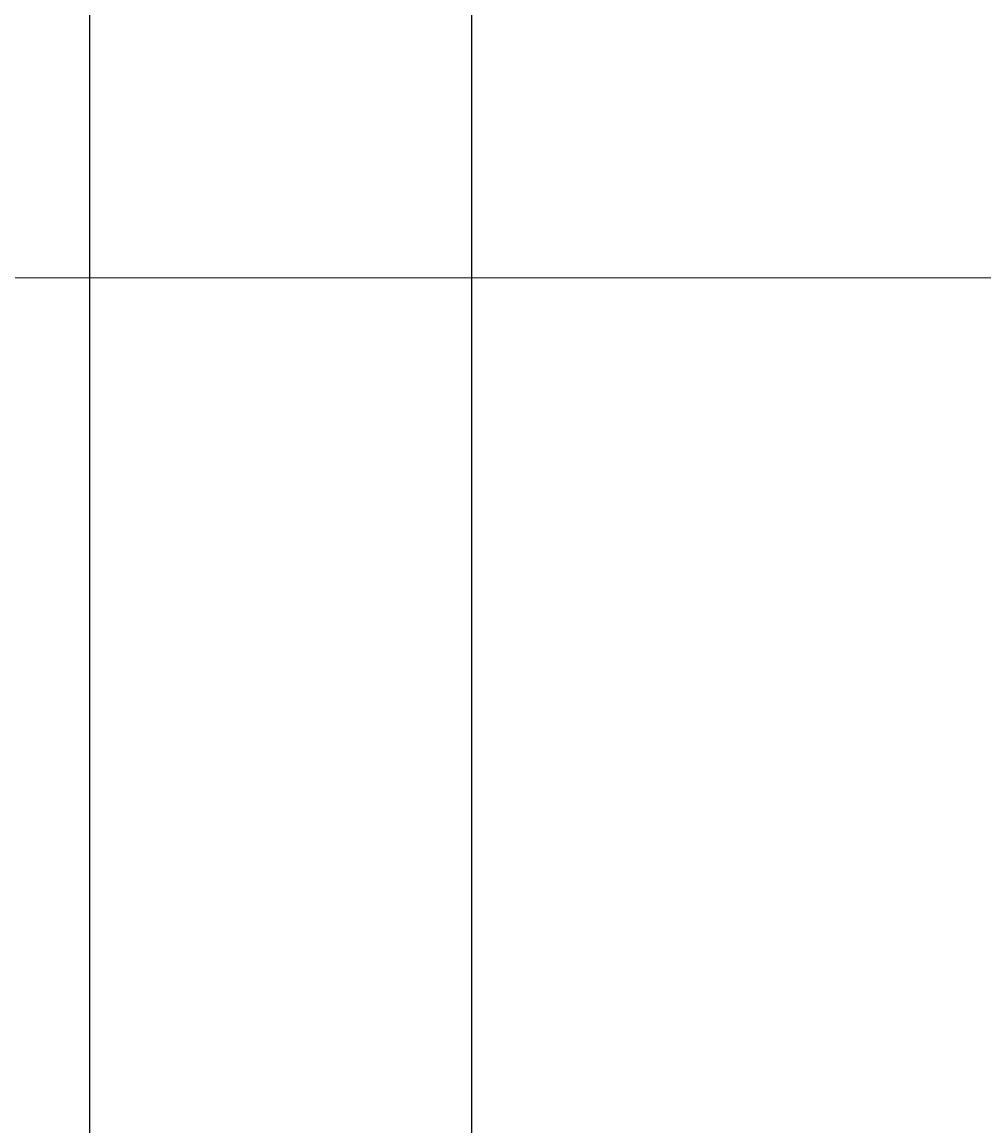
# Model space of a CAD drawing. Units: inches. Extents: x 738 to 1068, y 378 to 757.
# Tile 30 of 41: x 833 to 882, y 549 to 606. Entities that reach past the tile are written whole.
import ezdxf

# ---------------------------------------------------------------- set-up
doc = ezdxf.new("R2010")
doc.units = ezdxf.units.IN
doc.header["$MEASUREMENT"] = 0
doc.layers.add('A-ANNO-DIMS', color=2, linetype='Continuous', lineweight=18)
doc.layers.add('E-CTRL-WIRE', color=7, linetype='Continuous', lineweight=18)
doc.styles.get("Standard").update_dxf_attribs({"font": 'arial.ttf'})
doc.dimstyles.get("Standard").update_dxf_attribs({"dimtxt": 0.18, "dimasz": 0.18, "dimexe": 0.18, "dimexo": 0.0625, "dimgap": 0.09, "dimtad": 0, "dimtih": 1, "dimtoh": 1, "dimdec": 4, "dimzin": 0, "dimdsep": 46, "dimtxsty": 'Standard', "dimcen": 0.09, "dimadec": 0, "dimazin": 0, "dimtfac": 1, "dimtdec": 4, "dimtofl": 0, "dimtmove": 0, "dimatfit": 3, "dimfxl": 1, "dimtolj": 1, "dimtzin": 0, "dimarcsym": 0})

# ---------------------------------------------------------------- blocks, each defined once
blk = doc.blocks.new('*D32')
at = {"layer": 'A-ANNO-DIMS', "color": 0, "lineweight": -2, "transparency": 16777216}
for p, q in [((809.38, 461.454), (809.38, 756.505)), ((809.56, 756.325), (822.41, 756.325)), ((836.052, 756.325), (823.202, 756.325)), ((836.232, 461.277), (836.232, 756.505))]:
    blk.add_line(p, q, dxfattribs=at)
at = {"layer": 'A-ANNO-DIMS', "color": 0, "transparency": 16777216}
for points in [[(809.56, 756.355), (809.56, 756.295), (809.38, 756.325)], [(836.052, 756.355), (836.052, 756.295), (836.232, 756.325)]]:
    blk.add_solid(points, dxfattribs=at)
at = {"layer": 'Defpoints', "color": 0, "transparency": 16777216}
for p in [(836.232, 756.325), (809.38, 461.392), (836.232, 461.214)]:
    blk.add_point(p, dxfattribs=at)
at = {"layer": 'A-ANNO-DIMS', "color": 0, "transparency": 16777216, "insert": (822.806, 756.325), "char_height": 0.18, "attachment_point": 5}
blk.add_mtext('\\A1;26.85', dxfattribs=at)
blk = doc.blocks.new('*D35')
at = {"layer": 'A-ANNO-DIMS', "color": 0, "lineweight": -2, "transparency": 16777216}
for p, q in [((855.932, 686.266), (855.932, 378.239)), ((901.429, 686.267), (901.429, 378.239)), ((856.112, 378.419), (878.352, 378.419)), ((901.249, 378.419), (879.009, 378.419))]:
    blk.add_line(p, q, dxfattribs=at)
at = {"layer": 'A-ANNO-DIMS', "color": 0, "transparency": 16777216}
for points in [[(856.112, 378.449), (856.112, 378.389), (855.932, 378.419)], [(901.249, 378.449), (901.249, 378.389), (901.429, 378.419)]]:
    blk.add_solid(points, dxfattribs=at)
at = {"layer": 'Defpoints', "color": 0, "transparency": 16777216}
for p in [(855.932, 686.329), (901.429, 686.329), (901.429, 378.419)]:
    blk.add_point(p, dxfattribs=at)
at = {"layer": 'A-ANNO-DIMS', "color": 0, "transparency": 16777216, "insert": (878.68, 378.419), "char_height": 0.18, "attachment_point": 5}
blk.add_mtext('\\A1;45.5', dxfattribs=at)
blk = doc.blocks.new('*D38')
at = {"layer": 'A-ANNO-DIMS', "color": 0, "lineweight": -2, "transparency": 16777216}
for p, q in [((781.485, 593.017), (781.485, 378.239)), ((887.04, 593.067), (887.04, 378.239)), ((781.665, 378.419), (833.807, 378.419)), ((886.86, 378.419), (834.718, 378.419))]:
    blk.add_line(p, q, dxfattribs=at)
at = {"layer": 'A-ANNO-DIMS', "color": 0, "transparency": 16777216}
for points in [[(781.665, 378.449), (781.665, 378.389), (781.485, 378.419)], [(886.86, 378.449), (886.86, 378.389), (887.04, 378.419)]]:
    blk.add_solid(points, dxfattribs=at)
at = {"layer": 'Defpoints', "color": 0, "transparency": 16777216}
for p in [(781.485, 593.08), (887.04, 593.13), (887.04, 378.419)]:
    blk.add_point(p, dxfattribs=at)
at = {"layer": 'A-ANNO-DIMS', "color": 0, "transparency": 16777216, "insert": (834.263, 378.419), "char_height": 0.18, "attachment_point": 5}
blk.add_mtext('\\A1;105.56', dxfattribs=at)

msp = doc.modelspace()

# ---------------------------------------------------------------- linework, layer by layer
at = {"layer": 'E-CTRL-WIRE'}
msp.add_line((781.4897, 593.1296), (887.0404, 593.1296), dxfattribs=at)

# ---------------------------------------------------------------- dimensions: what is measured, and where the dimension line sits
at = {"layer": 'A-ANNO-DIMS'}
for base, p1, p2, override, picture, middle in [((836.2324, 756.3251), (809.3803, 461.3919), (836.2324, 461.214), {"dimdec": 2, "dimlfac": 1, "dimrnd": 0, "dimzin": 0, "dimdsep": 46, "dimlunit": 2}, '*D32', (822.8064, 756.3251)), ((901.4286, 378.4191), (855.9323, 686.329), (901.4286, 686.3292), {"dimdec": 1, "dimlfac": 1, "dimrnd": 0, "dimzin": 0, "dimdsep": 46, "dimlunit": 2}, '*D35', (878.6804, 378.4191)), ((887.0404, 378.4191), (781.4846, 593.0796), (887.0404, 593.1296), {"dimdec": 2, "dimlfac": 1, "dimrnd": 0, "dimzin": 0, "dimdsep": 46, "dimlunit": 2}, '*D38', (834.2625, 378.4191))]:
    dim = msp.add_linear_dim(base=base, p1=p1, p2=p2, dimstyle='Standard', override=override, dxfattribs=at)
    dim.commit()
    dim.dimension.update_dxf_attribs({"geometry": picture, "text_midpoint": middle})

doc.saveas('drawing.dxf')
